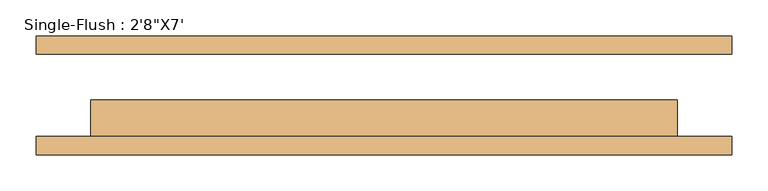
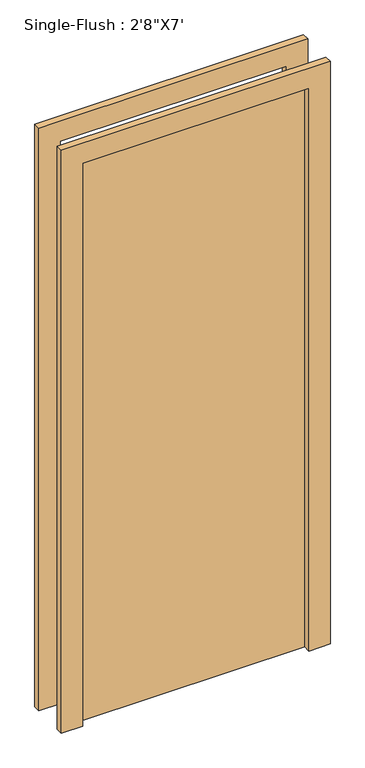
"""IFC4 building model written with IfcOpenShell, lengths in millimetres: door geometry."""

from ifc_helpers import new_model, si_unit, frame, origin, origin_with_axes, place, context, project, spatial, polyline, outline, extrude, source, transform, mapped, element, save


def door_38851409(model_context):
    return source(origin(), model_context, "Body", "SweptSolid", [
        extrude(outline(polyline([(2209.8, -482.6), (0.0, -482.6), (0.0, -406.4), (2133.6, -406.4), (2133.6, 406.4), (0.0, 406.4), (0.0, 482.6), (2209.8, 482.6), (2209.8, -482.6)])), frame((0.0, -82.55, 0.0), z_axis=(0.0, 1.0, 0.0), x_axis=(0.0, 0.0, 1.0)), (0.0, 0.0, 1.0), 25.4),
        extrude(outline(polyline([(2209.8, 482.6), (2209.8, -482.6), (0.0, -482.6), (0.0, -406.4), (2133.6, -406.4), (2133.6, 406.4), (0.0, 406.4), (0.0, 482.6), (2209.8, 482.6)])), frame((0.0, 57.15, 0.0), z_axis=(0.0, 1.0, 0.0), x_axis=(0.0, 0.0, 1.0)), (0.0, 0.0, 1.0), 25.4),
        extrude(outline(polyline([(406.4, -6.35), (406.4, -57.15), (-406.4, -57.15), (-406.4, -6.35), (406.4, -6.35)])), origin_with_axes(), (0.0, 0.0, 1.0), 2133.6),
    ])


if __name__ == "__main__":
    model = new_model("IFC4")
    model_context = context("Model", 3, world=origin())
    ifc_project = project(units=[si_unit("LENGTHUNIT", "METRE", prefix="MILLI")], contexts=[model_context])
    site = spatial("IfcSite", under=ifc_project)
    building = spatial("IfcBuilding", under=site)
    placement = place(None, origin())
    door_shape = door_38851409(model_context)
    element("IfcDoor", 1, ObjectType="Single-Flush : 2'8\"X7'", at=placement, inside=building, context=model_context, shape_type="MappedRepresentation", body=[
        mapped(door_shape, transform((0.0, 0.0, 0.0), x_axis=(1.0, 0.0, 0.0), y_axis=(0.0, 1.0, 0.0), z_axis=(0.0, 0.0, 1.0))),
    ])
    save(model, "model.ifc")

# Revit data of these elements
# Type "Single-Flush : 2'8\"X7'"
#   Type Mark = "12"
#   Construction Type Id = "MDOOR"
#   Assembly Code = "C1020"
#   Analytic Construction = "Metal"
#   Thickness = 0' - 2"
#   Heat Transfer Coefficient (U) = 0.651978 BTU/(h·ft²·°F)
#   Height = 7' - 0"
#   Trim Projection Ext = 0' - 1"
#   Trim Projection Int = 0' - 1"
#   Trim Width = 0' - 3"
#   Width = 2' - 8"
#   Define Thermal Properties by = 1
#   Door Material = Door - Panel
#   Frame Material = Door - Frame
#   Visual Light Transmittance = 0
#   Solar Heat Gain Coefficient = 0
#   Function = (empty or 0)
#   Wall Closure = (empty or 0)
# Element 1 (IfcDoor, "Single-Flush : 2'8\"X7'")
#   Materials on its faces: "Door - Frame", "Door - Panel"
# Materials
#   "Door - Panel": class "Wood", colour RGB 210 159 95, transparency 0, Cost = 0
#   "Door - Frame": colour RGB 118 70 51, transparency 0, Cost = 0
